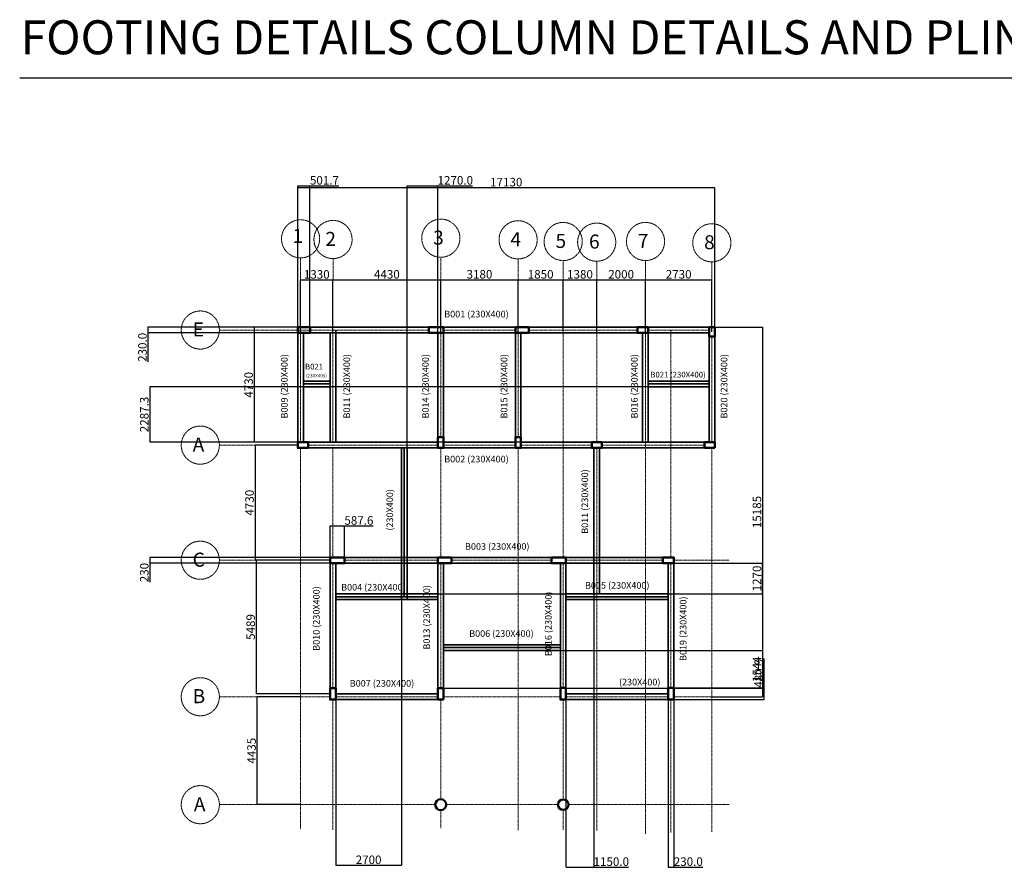
# Model space of a CAD drawing. Units: millimetres. Extents: x -2405 to 73447, y 417 to 55353.
# Tile 2 of 3: x -2405 to 38054, y 20479 to 55353. Entities that reach past the tile are written whole.
import ezdxf

# ---------------------------------------------------------------- set-up
doc = ezdxf.new("R2010")
doc.units = ezdxf.units.MM
doc.linetypes.add('CENTER', pattern=[50.8, 31.75, -6.35, 6.35, -6.35])
for name, color, linetype, lineweight in [('S-ANNO-DIMS', 2, 'Continuous', 18), ('S-ANNO-TEXT', 7, 'Continuous', 25), ('S-BEAM', 7, 'Continuous', 35), ('S-COLS', 4, 'Continuous', 50), ('S-GRID', 1, 'CENTER', 18)]:
    doc.layers.add(name, color=color, linetype=linetype, lineweight=lineweight)
doc.styles.get("Standard").update_dxf_attribs({"font": 'arial.ttf'})
doc.dimstyles.new('ISO-25', dxfattribs={"dimtxt": 350, "dimasz": 2.5, "dimexe": 1.25, "dimexo": 0.625, "dimtad": 1, "dimdec": 0, "dimtxsty": 'Standard', "dimcen": 2.5, "dimadec": 0, "dimazin": 0, "dimtfac": 1, "dimtdec": 0, "dimtmove": 0, "dimatfit": 3, "dimfxl": 1, "dimarcsym": 0})

# ---------------------------------------------------------------- blocks, each defined once
blk = doc.blocks.new('*D1')
at = {"layer": 'Defpoints', "color": 0, "transparency": 16777216}
for p in [(9023, 42715), (7229, 37985), (9023, 37985)]:
    blk.add_point(p, dxfattribs=at)
at = {"layer": 'S-ANNO-DIMS', "color": 0, "lineweight": -2, "transparency": 16777216}
for p, q in [((9022, 42715), (7227, 42715)), ((7229, 42712), (7229, 37987)), ((9022, 37985), (7227, 37985))]:
    blk.add_line(p, q, dxfattribs=at)
at = {"layer": 'S-ANNO-DIMS', "color": 0, "transparency": 16777216}
for points in [[(7228, 42712), (7229, 42712), (7229, 42715)], [(7228, 37987), (7229, 37987), (7229, 37985)]]:
    blk.add_solid(points, dxfattribs=at)
at = {"layer": 'S-ANNO-DIMS', "color": 0, "transparency": 16777216, "insert": (7049, 40350), "char_height": 350, "attachment_point": 5, "rotation": 90}
blk.add_mtext('4730', dxfattribs=at)
blk = doc.blocks.new('*D2')
at = {"layer": 'Defpoints', "color": 0, "transparency": 16777216}
for p in [(9023, 37870), (7265, 33140), (9138, 33140)]:
    blk.add_point(p, dxfattribs=at)
at = {"layer": 'S-ANNO-DIMS', "color": 0, "lineweight": -2, "transparency": 16777216}
for p, q in [((9022, 37870), (7263, 37870)), ((7265, 37867), (7265, 33142)), ((9137, 33140), (7263, 33140))]:
    blk.add_line(p, q, dxfattribs=at)
at = {"layer": 'S-ANNO-DIMS', "color": 0, "transparency": 16777216}
for points in [[(7264, 37867), (7265, 37867), (7265, 37870)], [(7264, 33142), (7265, 33142), (7265, 33140)]]:
    blk.add_solid(points, dxfattribs=at)
at = {"layer": 'S-ANNO-DIMS', "color": 0, "transparency": 16777216, "insert": (7085, 35505), "char_height": 350, "attachment_point": 5, "rotation": 90}
blk.add_mtext('4730', dxfattribs=at)
blk = doc.blocks.new('*D3')
at = {"layer": 'Defpoints', "color": 0, "transparency": 16777216}
for p in [(10353, 33140), (7309, 27651), (10353, 27651)]:
    blk.add_point(p, dxfattribs=at)
at = {"layer": 'S-ANNO-DIMS', "color": 0, "lineweight": -2, "transparency": 16777216}
for p, q in [((10352, 33140), (7308, 33140)), ((7309, 33137), (7309, 27654)), ((10352, 27651), (7308, 27651))]:
    blk.add_line(p, q, dxfattribs=at)
at = {"layer": 'S-ANNO-DIMS', "color": 0, "transparency": 16777216}
for points in [[(7309, 33137), (7310, 33137), (7309, 33140)], [(7309, 27654), (7310, 27654), (7309, 27651)]]:
    blk.add_solid(points, dxfattribs=at)
at = {"layer": 'S-ANNO-DIMS', "color": 0, "transparency": 16777216, "insert": (7130, 30396), "char_height": 350, "attachment_point": 5, "rotation": 90}
blk.add_mtext('5489', dxfattribs=at)
blk = doc.blocks.new('*D4')
at = {"layer": 'Defpoints', "color": 0, "transparency": 16777216}
for p in [(9138, 27530), (7345, 23095), (9138, 23095)]:
    blk.add_point(p, dxfattribs=at)
at = {"layer": 'S-ANNO-DIMS', "color": 0, "lineweight": -2, "transparency": 16777216}
for p, q in [((9137, 27530), (7344, 27530)), ((7345, 27527), (7345, 23097)), ((9137, 23095), (7344, 23095))]:
    blk.add_line(p, q, dxfattribs=at)
at = {"layer": 'S-ANNO-DIMS', "color": 0, "transparency": 16777216}
for points in [[(7345, 27527), (7346, 27527), (7345, 27530)], [(7345, 23097), (7346, 23097), (7345, 23095)]]:
    blk.add_solid(points, dxfattribs=at)
at = {"layer": 'S-ANNO-DIMS', "color": 0, "transparency": 16777216, "insert": (7166, 25312), "char_height": 350, "attachment_point": 5, "rotation": 90}
blk.add_mtext('4435', dxfattribs=at)
blk = doc.blocks.new('*D5')
at = {"layer": 'Defpoints', "color": 0, "transparency": 16777216}
for p in [(10468, 44661), (9138, 42485), (10468, 42485)]:
    blk.add_point(p, dxfattribs=at)
at = {"layer": 'S-ANNO-DIMS', "color": 0, "lineweight": -2, "transparency": 16777216}
for p, q in [((9138, 42486), (9138, 44662)), ((9140, 44661), (10465, 44661)), ((10468, 42486), (10468, 44662))]:
    blk.add_line(p, q, dxfattribs=at)
at = {"layer": 'S-ANNO-DIMS', "color": 0, "transparency": 16777216}
for points in [[(9140, 44662), (9140, 44661), (9138, 44661)], [(10465, 44662), (10465, 44661), (10468, 44661)]]:
    blk.add_solid(points, dxfattribs=at)
at = {"layer": 'S-ANNO-DIMS', "color": 0, "transparency": 16777216, "insert": (9803, 44841), "char_height": 350, "attachment_point": 5}
blk.add_mtext('1330', dxfattribs=at)
blk = doc.blocks.new('*D6')
at = {"layer": 'Defpoints', "color": 0, "transparency": 16777216}
for p in [(14898, 44665), (10468, 42485), (14898, 42485)]:
    blk.add_point(p, dxfattribs=at)
at = {"layer": 'S-ANNO-DIMS', "color": 0, "lineweight": -2, "transparency": 16777216}
for p, q in [((10468, 42486), (10468, 44666)), ((10470, 44665), (14895, 44665)), ((14898, 42486), (14898, 44666))]:
    blk.add_line(p, q, dxfattribs=at)
at = {"layer": 'S-ANNO-DIMS', "color": 0, "transparency": 16777216}
for points in [[(10470, 44665), (10470, 44664), (10468, 44665)], [(14895, 44665), (14895, 44664), (14898, 44665)]]:
    blk.add_solid(points, dxfattribs=at)
at = {"layer": 'S-ANNO-DIMS', "color": 0, "transparency": 16777216, "insert": (12683, 44844), "char_height": 350, "attachment_point": 5}
blk.add_mtext('4430', dxfattribs=at)
blk = doc.blocks.new('*D7')
at = {"layer": 'Defpoints', "color": 0, "transparency": 16777216}
for p in [(18078, 44666), (14898, 42485), (18078, 42485)]:
    blk.add_point(p, dxfattribs=at)
at = {"layer": 'S-ANNO-DIMS', "color": 0, "lineweight": -2, "transparency": 16777216}
for p, q in [((14898, 42486), (14898, 44667)), ((14900, 44666), (18075, 44666)), ((18078, 42486), (18078, 44667))]:
    blk.add_line(p, q, dxfattribs=at)
at = {"layer": 'S-ANNO-DIMS', "color": 0, "transparency": 16777216}
for points in [[(14900, 44667), (14900, 44666), (14898, 44666)], [(18075, 44667), (18075, 44666), (18078, 44666)]]:
    blk.add_solid(points, dxfattribs=at)
at = {"layer": 'S-ANNO-DIMS', "color": 0, "transparency": 16777216, "insert": (16488, 44846), "char_height": 350, "attachment_point": 5}
blk.add_mtext('3180', dxfattribs=at)
blk = doc.blocks.new('*D8')
at = {"layer": 'Defpoints', "color": 0, "transparency": 16777216}
for p in [(19928, 44666), (18078, 42485), (19928, 42600)]:
    blk.add_point(p, dxfattribs=at)
at = {"layer": 'S-ANNO-DIMS', "color": 0, "lineweight": -2, "transparency": 16777216}
for p, q in [((18078, 42486), (18078, 44667)), ((18080, 44666), (19925, 44666)), ((19928, 42601), (19928, 44667))]:
    blk.add_line(p, q, dxfattribs=at)
at = {"layer": 'S-ANNO-DIMS', "color": 0, "transparency": 16777216}
for points in [[(18080, 44666), (18080, 44665), (18078, 44666)], [(19925, 44666), (19925, 44665), (19928, 44666)]]:
    blk.add_solid(points, dxfattribs=at)
at = {"layer": 'S-ANNO-DIMS', "color": 0, "transparency": 16777216, "insert": (19003, 44845), "char_height": 350, "attachment_point": 5}
blk.add_mtext('1850', dxfattribs=at)
blk = doc.blocks.new('*D9')
at = {"layer": 'Defpoints', "color": 0, "transparency": 16777216}
for p in [(21308, 44666), (19928, 42600), (21308, 42485)]:
    blk.add_point(p, dxfattribs=at)
at = {"layer": 'S-ANNO-DIMS', "color": 0, "lineweight": -2, "transparency": 16777216}
for p, q in [((19928, 42601), (19928, 44667)), ((19930, 44666), (21305, 44666)), ((21308, 42486), (21308, 44667))]:
    blk.add_line(p, q, dxfattribs=at)
at = {"layer": 'S-ANNO-DIMS', "color": 0, "transparency": 16777216}
for points in [[(19930, 44666), (19930, 44665), (19928, 44666)], [(21305, 44666), (21305, 44665), (21308, 44666)]]:
    blk.add_solid(points, dxfattribs=at)
at = {"layer": 'S-ANNO-DIMS', "color": 0, "transparency": 16777216, "insert": (20618, 44845), "char_height": 350, "attachment_point": 5}
blk.add_mtext('1380', dxfattribs=at)
blk = doc.blocks.new('*D10')
at = {"layer": 'Defpoints', "color": 0, "transparency": 16777216}
for p in [(23308, 44665), (21308, 42600), (23308, 42485)]:
    blk.add_point(p, dxfattribs=at)
at = {"layer": 'S-ANNO-DIMS', "color": 0, "lineweight": -2, "transparency": 16777216}
for p, q in [((21308, 42601), (21308, 44667)), ((21310, 44665), (23305, 44665)), ((23308, 42486), (23308, 44667))]:
    blk.add_line(p, q, dxfattribs=at)
at = {"layer": 'S-ANNO-DIMS', "color": 0, "transparency": 16777216}
for points in [[(21310, 44666), (21310, 44665), (21308, 44665)], [(23305, 44666), (23305, 44665), (23308, 44665)]]:
    blk.add_solid(points, dxfattribs=at)
at = {"layer": 'S-ANNO-DIMS', "color": 0, "transparency": 16777216, "insert": (22308, 44845), "char_height": 350, "attachment_point": 5}
blk.add_mtext('2000', dxfattribs=at)
blk = doc.blocks.new('*D11')
at = {"layer": 'Defpoints', "color": 0, "transparency": 16777216}
for p in [(26038, 44666), (23308, 42485), (26038, 42525)]:
    blk.add_point(p, dxfattribs=at)
at = {"layer": 'S-ANNO-DIMS', "color": 0, "lineweight": -2, "transparency": 16777216}
for p, q in [((23308, 42486), (23308, 44667)), ((23310, 44666), (26035, 44666)), ((26038, 42525), (26038, 44667))]:
    blk.add_line(p, q, dxfattribs=at)
at = {"layer": 'S-ANNO-DIMS', "color": 0, "transparency": 16777216}
for points in [[(23310, 44666), (23310, 44665), (23308, 44666)], [(26035, 44666), (26035, 44665), (26038, 44666)]]:
    blk.add_solid(points, dxfattribs=at)
at = {"layer": 'S-ANNO-DIMS', "color": 0, "transparency": 16777216, "insert": (24673, 44845), "char_height": 350, "attachment_point": 5}
blk.add_mtext('2730', dxfattribs=at)
blk = doc.blocks.new('*D14')
at = {"layer": 'Defpoints', "color": 0, "transparency": 16777216}
for p in [(26153, 48453), (9023, 42715), (26153, 42715)]:
    blk.add_point(p, dxfattribs=at)
at = {"layer": 'S-ANNO-DIMS', "color": 0, "lineweight": -2, "transparency": 16777216}
for p, q in [((9023, 42716), (9023, 48454)), ((9025, 48453), (26150, 48453)), ((26153, 42716), (26153, 48454))]:
    blk.add_line(p, q, dxfattribs=at)
at = {"layer": 'S-ANNO-DIMS', "color": 0, "transparency": 16777216}
for points in [[(9025, 48453), (9025, 48452), (9023, 48453)], [(26150, 48453), (26150, 48452), (26153, 48453)]]:
    blk.add_solid(points, dxfattribs=at)
at = {"layer": 'S-ANNO-DIMS', "color": 0, "transparency": 16777216, "insert": (17588, 48632), "char_height": 350, "attachment_point": 5}
blk.add_mtext('17130', dxfattribs=at)
blk = doc.blocks.new('*D15')
at = {"layer": 'Defpoints', "color": 0, "transparency": 16777216}
for p in [(26153, 42715), (26038, 27530), (28113, 27530)]:
    blk.add_point(p, dxfattribs=at)
at = {"layer": 'S-ANNO-DIMS', "color": 0, "lineweight": -2, "transparency": 16777216}
for p, q in [((26153, 42715), (28115, 42715)), ((28113, 42712), (28113, 27532)), ((26038, 27530), (28115, 27530))]:
    blk.add_line(p, q, dxfattribs=at)
at = {"layer": 'S-ANNO-DIMS', "color": 0, "transparency": 16777216}
for points in [[(28113, 42712), (28114, 42712), (28113, 42715)], [(28113, 27532), (28114, 27532), (28113, 27530)]]:
    blk.add_solid(points, dxfattribs=at)
at = {"layer": 'S-ANNO-DIMS', "color": 0, "transparency": 16777216, "insert": (27934, 35122), "char_height": 350, "attachment_point": 5, "rotation": 90}
blk.add_mtext('15185', dxfattribs=at)
blk = doc.blocks.new('*D16')
at = {"layer": 'Defpoints', "color": 0, "transparency": 16777216}
for p in [(10940, 34550), (10353, 33255), (10940, 33255)]:
    blk.add_point(p, dxfattribs=at)
at = {"layer": 'S-ANNO-DIMS', "color": 0, "lineweight": -2, "transparency": 16777216}
for p, q in [((10353, 33256), (10353, 34551)), ((10355, 34550), (10938, 34550)), ((10940, 33256), (10940, 34551)), ((10940, 34550), (12125, 34550))]:
    blk.add_line(p, q, dxfattribs=at)
at = {"layer": 'S-ANNO-DIMS', "color": 0, "transparency": 16777216}
for points in [[(10355, 34550), (10355, 34550), (10353, 34550)], [(10938, 34550), (10938, 34550), (10940, 34550)]]:
    blk.add_solid(points, dxfattribs=at)
at = {"layer": 'S-ANNO-DIMS', "color": 0, "transparency": 16777216, "insert": (11534, 34729), "char_height": 350, "attachment_point": 5}
blk.add_mtext('587.6', dxfattribs=at)
blk = doc.blocks.new('*D17')
at = {"layer": 'Defpoints', "color": 0, "transparency": 16777216}
for p in [(14783, 33255), (2939, 33025), (14783, 33025)]:
    blk.add_point(p, dxfattribs=at)
at = {"layer": 'S-ANNO-DIMS', "color": 0, "lineweight": -2, "transparency": 16777216}
for p, q in [((14782, 33255), (2938, 33255)), ((2939, 33252), (2939, 33027)), ((14782, 33025), (2938, 33025)), ((2939, 33025), (2939, 32243))]:
    blk.add_line(p, q, dxfattribs=at)
at = {"layer": 'S-ANNO-DIMS', "color": 0, "transparency": 16777216}
for points in [[(2939, 33252), (2940, 33252), (2939, 33255)], [(2939, 33027), (2940, 33027), (2939, 33025)]]:
    blk.add_solid(points, dxfattribs=at)
at = {"layer": 'S-ANNO-DIMS', "color": 0, "transparency": 16777216, "insert": (2760, 32633), "char_height": 350, "attachment_point": 5, "rotation": 90}
blk.add_mtext('230', dxfattribs=at)
blk = doc.blocks.new('*D18')
at = {"layer": 'Defpoints', "color": 0, "transparency": 16777216}
for p in [(10583, 31525), (13283, 31525), (13283, 20604)]:
    blk.add_point(p, dxfattribs=at)
at = {"layer": 'S-ANNO-DIMS', "color": 0, "lineweight": -2, "transparency": 16777216}
for p, q in [((10583, 31524), (10583, 20603)), ((13283, 31524), (13283, 20603)), ((10585, 20604), (13280, 20604))]:
    blk.add_line(p, q, dxfattribs=at)
at = {"layer": 'S-ANNO-DIMS', "color": 0, "transparency": 16777216}
for points in [[(10585, 20605), (10585, 20604), (10583, 20604)], [(13280, 20605), (13280, 20604), (13283, 20604)]]:
    blk.add_solid(points, dxfattribs=at)
at = {"layer": 'S-ANNO-DIMS', "color": 0, "transparency": 16777216, "insert": (11933, 20784), "char_height": 350, "attachment_point": 5}
blk.add_mtext('2700', dxfattribs=at)
blk = doc.blocks.new('*D19')
at = {"layer": 'Defpoints', "color": 0, "transparency": 16777216}
for p in [(14783, 33025), (28113, 33025), (14783, 31755)]:
    blk.add_point(p, dxfattribs=at)
at = {"layer": 'S-ANNO-DIMS', "color": 0, "lineweight": -2, "transparency": 16777216}
for p, q in [((14783, 33025), (28115, 33025)), ((28113, 31757), (28113, 33022)), ((14783, 31755), (28115, 31755))]:
    blk.add_line(p, q, dxfattribs=at)
at = {"layer": 'S-ANNO-DIMS', "color": 0, "transparency": 16777216}
for points in [[(28113, 33022), (28114, 33022), (28113, 33025)], [(28113, 31757), (28114, 31757), (28113, 31755)]]:
    blk.add_solid(points, dxfattribs=at)
at = {"layer": 'S-ANNO-DIMS', "color": 0, "transparency": 16777216, "insert": (27934, 32390), "char_height": 350, "attachment_point": 5, "rotation": 90}
blk.add_mtext('1270', dxfattribs=at)
blk = doc.blocks.new('*D20')
at = {"layer": 'Defpoints', "color": 0, "transparency": 16777216}
for p in [(15013, 29432), (15013, 27888), (28113, 27888)]:
    blk.add_point(p, dxfattribs=at)
at = {"layer": 'S-ANNO-DIMS', "color": 0, "lineweight": -2, "transparency": 16777216}
for p, q in [((15013, 29432), (28115, 29432)), ((28113, 29429), (28113, 27890)), ((15013, 27888), (28115, 27888))]:
    blk.add_line(p, q, dxfattribs=at)
at = {"layer": 'S-ANNO-DIMS', "color": 0, "transparency": 16777216}
for points in [[(28113, 29429), (28114, 29429), (28113, 29432)], [(28113, 27890), (28114, 27890), (28113, 27888)]]:
    blk.add_solid(points, dxfattribs=at)
at = {"layer": 'S-ANNO-DIMS', "color": 0, "transparency": 16777216, "insert": (27934, 28660), "char_height": 350, "attachment_point": 5, "rotation": 90}
blk.add_mtext('1544', dxfattribs=at)
blk = doc.blocks.new('*D21')
at = {"layer": 'Defpoints', "color": 0, "transparency": 16777216}
for p in [(25923, 40272), (2939, 37985), (25923, 37985)]:
    blk.add_point(p, dxfattribs=at)
at = {"layer": 'S-ANNO-DIMS', "color": 0, "lineweight": -2, "transparency": 16777216}
for p, q in [((25922, 40272), (2938, 40272)), ((2939, 40270), (2939, 37987)), ((25922, 37985), (2938, 37985))]:
    blk.add_line(p, q, dxfattribs=at)
at = {"layer": 'S-ANNO-DIMS', "color": 0, "transparency": 16777216}
for points in [[(2939, 40270), (2940, 40270), (2939, 40272)], [(2939, 37987), (2940, 37987), (2939, 37985)]]:
    blk.add_solid(points, dxfattribs=at)
at = {"layer": 'S-ANNO-DIMS', "color": 0, "transparency": 16777216, "insert": (2760, 39129), "char_height": 350, "attachment_point": 5, "rotation": 90}
blk.add_mtext('2287.3', dxfattribs=at)
blk = doc.blocks.new('*D22')
at = {"layer": 'Defpoints', "color": 0, "transparency": 16777216}
for p in [(24358, 33025), (28113, 33025), (24243, 31755)]:
    blk.add_point(p, dxfattribs=at)
at = {"layer": 'S-ANNO-DIMS', "color": 0, "lineweight": -2, "transparency": 16777216}
for p, q in [((24358, 33025), (28115, 33025)), ((28113, 31757), (28113, 33022)), ((24243, 31755), (28115, 31755))]:
    blk.add_line(p, q, dxfattribs=at)
at = {"layer": 'S-ANNO-DIMS', "color": 0, "transparency": 16777216}
for points in [[(28113, 33022), (28114, 33022), (28113, 33025)], [(28113, 31757), (28114, 31757), (28113, 31755)]]:
    blk.add_solid(points, dxfattribs=at)
at = {"layer": 'S-ANNO-DIMS', "color": 0, "transparency": 16777216, "insert": (27934, 32390), "char_height": 350, "attachment_point": 5, "rotation": 90}
blk.add_mtext('1270', dxfattribs=at)
blk = doc.blocks.new('*D40')
at = {"layer": 'Defpoints', "color": 0, "transparency": 16777216}
for p in [(9524, 48528), (9023, 42715), (9524, 42715)]:
    blk.add_point(p, dxfattribs=at)
at = {"layer": 'S-ANNO-DIMS', "color": 0, "lineweight": -2, "transparency": 16777216}
for p, q in [((9023, 42716), (9023, 48529)), ((9025, 48528), (9522, 48528)), ((9524, 42716), (9524, 48529)), ((9524, 48528), (10709, 48528))]:
    blk.add_line(p, q, dxfattribs=at)
at = {"layer": 'S-ANNO-DIMS', "color": 0, "transparency": 16777216}
for points in [[(9025, 48528), (9025, 48527), (9023, 48528)], [(9522, 48528), (9522, 48527), (9524, 48528)]]:
    blk.add_solid(points, dxfattribs=at)
at = {"layer": 'S-ANNO-DIMS', "color": 0, "transparency": 16777216, "insert": (10118, 48707), "char_height": 350, "attachment_point": 5}
blk.add_mtext('501.7', dxfattribs=at)
blk = doc.blocks.new('*D41')
at = {"layer": 'Defpoints', "color": 0, "transparency": 16777216}
for p in [(2864, 42485), (9023, 42715), (9023, 42485)]:
    blk.add_point(p, dxfattribs=at)
at = {"layer": 'S-ANNO-DIMS', "color": 0, "lineweight": -2, "transparency": 16777216}
for p, q in [((9022, 42715), (2863, 42715)), ((9022, 42485), (2863, 42485)), ((2864, 42712), (2864, 42487)), ((2864, 42485), (2864, 41295))]:
    blk.add_line(p, q, dxfattribs=at)
at = {"layer": 'S-ANNO-DIMS', "color": 0, "transparency": 16777216}
for points in [[(2864, 42712), (2865, 42712), (2864, 42715)], [(2864, 42487), (2865, 42487), (2864, 42485)]]:
    blk.add_solid(points, dxfattribs=at)
at = {"layer": 'S-ANNO-DIMS', "color": 0, "transparency": 16777216, "insert": (2685, 41889), "char_height": 350, "attachment_point": 5, "rotation": 90}
blk.add_mtext('230.0', dxfattribs=at)
blk = doc.blocks.new('*D42')
at = {"layer": 'Defpoints', "color": 0, "transparency": 16777216}
for p in [(24473, 27896), (28188, 27896), (24473, 27415)]:
    blk.add_point(p, dxfattribs=at)
at = {"layer": 'S-ANNO-DIMS', "color": 0, "lineweight": -2, "transparency": 16777216}
for p, q in [((28188, 27896), (28188, 29095)), ((24473, 27896), (28190, 27896)), ((28188, 27417), (28188, 27893)), ((24473, 27415), (28190, 27415))]:
    blk.add_line(p, q, dxfattribs=at)
at = {"layer": 'S-ANNO-DIMS', "color": 0, "transparency": 16777216}
for points in [[(28188, 27893), (28189, 27893), (28188, 27896)], [(28188, 27417), (28189, 27417), (28188, 27415)]]:
    blk.add_solid(points, dxfattribs=at)
at = {"layer": 'S-ANNO-DIMS', "color": 0, "transparency": 16777216, "insert": (28009, 28497), "char_height": 350, "attachment_point": 5, "rotation": 90}
blk.add_mtext('480.9', dxfattribs=at)
blk = doc.blocks.new('*D43')
at = {"layer": 'Defpoints', "color": 0, "transparency": 16777216}
for p in [(24243, 27415), (24473, 27415), (24473, 20529)]:
    blk.add_point(p, dxfattribs=at)
at = {"layer": 'S-ANNO-DIMS', "color": 0, "lineweight": -2, "transparency": 16777216}
for p, q in [((24243, 27414), (24243, 20528)), ((24473, 27414), (24473, 20528)), ((24245, 20529), (24470, 20529)), ((24473, 20529), (25662, 20529))]:
    blk.add_line(p, q, dxfattribs=at)
at = {"layer": 'S-ANNO-DIMS', "color": 0, "transparency": 16777216}
for points in [[(24245, 20530), (24245, 20529), (24243, 20529)], [(24470, 20530), (24470, 20529), (24473, 20529)]]:
    blk.add_solid(points, dxfattribs=at)
at = {"layer": 'S-ANNO-DIMS', "color": 0, "transparency": 16777216, "insert": (25069, 20709), "char_height": 350, "attachment_point": 5}
blk.add_mtext('230.0', dxfattribs=at)
blk = doc.blocks.new('*D44')
at = {"layer": 'Defpoints', "color": 0, "transparency": 16777216}
for p in [(14783, 48528), (13513, 37755), (14783, 37755)]:
    blk.add_point(p, dxfattribs=at)
at = {"layer": 'S-ANNO-DIMS', "color": 0, "lineweight": -2, "transparency": 16777216}
for p, q in [((13513, 37756), (13513, 48529)), ((13515, 48528), (14780, 48528)), ((14783, 37756), (14783, 48529)), ((14783, 48528), (16205, 48528))]:
    blk.add_line(p, q, dxfattribs=at)
at = {"layer": 'S-ANNO-DIMS', "color": 0, "transparency": 16777216}
for points in [[(13515, 48528), (13515, 48527), (13513, 48528)], [(14780, 48528), (14780, 48527), (14783, 48528)]]:
    blk.add_solid(points, dxfattribs=at)
at = {"layer": 'S-ANNO-DIMS', "color": 0, "transparency": 16777216, "insert": (15495, 48707), "char_height": 350, "attachment_point": 5}
blk.add_mtext('1270.0', dxfattribs=at)
blk = doc.blocks.new('*D45')
at = {"layer": 'Defpoints', "color": 0, "transparency": 16777216}
for p in [(20043, 31755), (21193, 31755), (21193, 20529)]:
    blk.add_point(p, dxfattribs=at)
at = {"layer": 'S-ANNO-DIMS', "color": 0, "lineweight": -2, "transparency": 16777216}
for p, q in [((20043, 31754), (20043, 20528)), ((21193, 31754), (21193, 20528)), ((20045, 20529), (21190, 20529)), ((21193, 20529), (22615, 20529))]:
    blk.add_line(p, q, dxfattribs=at)
at = {"layer": 'S-ANNO-DIMS', "color": 0, "transparency": 16777216}
for points in [[(20045, 20530), (20045, 20529), (20043, 20529)], [(21190, 20530), (21190, 20529), (21193, 20529)]]:
    blk.add_solid(points, dxfattribs=at)
at = {"layer": 'S-ANNO-DIMS', "color": 0, "transparency": 16777216, "insert": (21905, 20709), "char_height": 350, "attachment_point": 5}
blk.add_mtext('1150.0', dxfattribs=at)

msp = doc.modelspace()

# ---------------------------------------------------------------- linework, layer by layer
at = {"layer": 'S-ANNO-TEXT'}
msp.add_line((-2404.637, 52969.195), (57098.008, 52969.195), dxfattribs=at)
at = {"layer": 'S-BEAM'}
for p, q in [((9022.761, 42599.973), (9022.761, 42714.973)), ((9022.761, 42714.973), (9137.761, 42714.973)), ((9022.761, 42599.973), (9022.761, 37754.973)), ((9022.761, 42484.973), (10467.761, 42484.973)), ((9137.761, 42714.973), (10467.761, 42714.973)), ((9252.761, 42484.973), (9252.761, 37984.973)), ((10352.761, 42484.973), (10352.761, 37984.973)), ((10467.761, 42714.973), (14897.761, 42714.973)), ((10467.761, 42484.973), (14897.761, 42484.973)), ((10582.761, 42599.973), (10582.761, 37984.973)), ((14782.761, 42484.973), (14782.761, 37754.973)), ((14897.761, 42714.973), (18077.761, 42714.973)), ((14897.761, 42484.973), (18077.761, 42484.973)), ((15012.761, 42484.973), (15012.761, 37754.973)), ((17962.761, 42714.973), (17962.761, 37754.973)), ((18077.761, 42714.973), (19927.761, 42714.973)), ((18077.761, 42484.973), (19927.761, 42484.973)), ((18192.761, 42484.973), (18192.761, 37754.973)), ((19927.761, 42714.973), (21307.761, 42714.973)), ((19927.761, 42484.973), (21307.761, 42484.973)), ((21307.761, 42714.973), (23307.761, 42714.973)), ((21307.761, 42484.973), (23307.761, 42484.973)), ((23192.761, 42484.973), (23192.761, 37984.973)), ((23307.761, 42714.973), (24357.761, 42714.973)), ((23307.761, 42484.973), (24357.761, 42484.973)), ((23422.761, 42599.973), (23422.761, 37984.973)), ((24357.761, 42714.973), (26037.761, 42714.973)), ((24357.761, 42484.973), (25922.761, 42484.973)), ((25922.761, 37984.973), (25922.761, 42599.973)), ((26152.761, 42714.973), (26037.761, 42714.973)), ((26152.761, 42599.973), (26152.761, 42714.973)), ((26152.761, 37754.973), (26152.761, 42599.973)), ((9252.761, 40502.295), (10352.761, 40502.295)), ((23422.761, 40502.295), (25922.761, 40502.295)), ((9252.761, 40387.295), (10352.761, 40387.295)), ((9252.761, 40272.295), (10352.761, 40272.295)), ((23422.761, 40387.295), (25922.761, 40387.295)), ((23422.761, 40272.295), (25922.761, 40272.295)), ((9022.761, 37984.973), (10467.761, 37984.973)), ((9022.761, 37754.973), (10467.761, 37754.973)), ((10467.761, 37984.973), (14782.761, 37984.973)), ((10467.761, 37754.973), (14897.761, 37754.973)), ((13282.761, 37754.973), (13282.761, 31524.973)), ((13397.761, 37754.973), (13397.761, 31639.973)), ((13512.761, 37754.973), (13512.761, 31524.973)), ((14897.761, 37754.973), (19927.761, 37754.973)), ((15012.761, 37984.973), (17962.761, 37984.973)), ((18192.761, 37984.973), (19927.761, 37984.973)), ((19927.761, 37984.973), (21307.761, 37984.973)), ((19927.761, 37754.973), (21307.761, 37754.973)), ((21192.761, 37754.973), (21192.761, 31754.973)), ((21307.761, 37984.973), (23307.761, 37984.973)), ((21307.761, 37754.973), (23307.761, 37754.973)), ((21422.761, 37754.973), (21422.761, 31754.973)), ((23307.761, 37984.973), (26152.761, 37984.973)), ((23307.761, 37754.973), (26152.761, 37754.973)), ((10352.761, 33254.973), (14897.761, 33254.973)), ((10352.761, 33254.973), (10352.761, 27414.973)), ((14782.761, 33254.973), (14782.761, 27414.973)), ((14897.761, 33254.973), (18077.761, 33254.973)), ((18077.761, 33254.973), (19927.761, 33254.973)), ((19812.761, 33254.973), (21307.761, 33254.973)), ((20042.761, 33254.973), (20042.761, 27529.973)), ((21307.761, 33254.973), (23307.761, 33254.973)), ((23307.761, 33254.973), (24472.761, 33254.973)), ((24472.761, 33254.973), (24472.761, 27414.973)), ((10352.761, 33024.973), (14897.761, 33024.973)), ((10582.761, 33024.973), (10582.761, 27414.973)), ((14897.761, 33024.973), (18077.761, 33024.973)), ((15012.761, 33024.973), (15012.761, 27414.973)), ((18077.761, 33024.973), (19927.761, 33024.973)), ((19812.761, 33024.973), (21307.761, 33024.973)), ((19812.761, 33024.973), (19812.761, 27529.973)), ((21307.761, 33024.973), (23307.761, 33024.973)), ((23307.761, 33024.973), (24472.761, 33024.973)), ((24242.761, 33024.973), (24242.761, 27414.973)), ((10582.761, 31754.973), (14782.761, 31754.973)), ((10582.761, 31639.973), (14782.761, 31639.973)), ((20042.761, 31754.973), (21307.761, 31754.973)), ((20042.761, 31639.973), (21307.761, 31639.973)), ((21307.761, 31754.973), (23307.761, 31754.973)), ((21307.761, 31639.973), (23307.761, 31639.973)), ((23307.761, 31754.973), (24242.761, 31754.973)), ((23307.761, 31639.973), (24242.761, 31639.973)), ((10582.761, 31524.973), (14782.761, 31524.973)), ((20042.761, 31524.973), (21307.761, 31524.973)), ((21307.761, 31524.973), (23307.761, 31524.973)), ((23307.761, 31524.973), (24242.761, 31524.973)), ((15012.761, 29661.949), (19812.761, 29661.949)), ((15012.761, 29546.949), (19812.761, 29546.949)), ((15012.761, 29431.949), (19812.761, 29431.949)), ((10582.761, 27644.973), (14782.761, 27644.973)), ((20042.761, 27644.973), (23307.761, 27644.973)), ((23307.761, 27644.973), (24242.761, 27644.973)), ((10352.761, 27414.973), (15012.761, 27414.973)), ((19927.761, 27414.973), (23307.761, 27414.973)), ((23307.761, 27414.973), (24472.761, 27414.973))]:
    msp.add_line(p, q, dxfattribs=at)
at = {"layer": 'S-COLS'}
for points in [[(9022.761, 42714.973), (9524.48, 42714.973), (9524.48, 42484.973), (9022.761, 42484.973)], [(15012.761, 42484.973), (14411.901, 42484.973), (14411.901, 42714.973), (15012.761, 42714.973)], [(17962.761, 42484.973), (18518.958, 42484.973), (18518.958, 42714.973), (17962.761, 42714.973)], [(23422.761, 42484.973), (22981.975, 42484.973), (22981.975, 42714.973), (23422.761, 42714.973)], [(25922.761, 42714.973), (26152.761, 42714.973), (26152.761, 42334.257), (25922.761, 42334.257)], [(14782.761, 38201.603), (15012.761, 38201.603), (15012.761, 37754.973), (14782.761, 37754.973)], [(17962.761, 38195.273), (18192.761, 38195.273), (18192.761, 37754.973), (17962.761, 37754.973)], [(9022.761, 37984.973), (9448.304, 37984.973), (9448.304, 37754.973), (9022.761, 37754.973)], [(21099.782, 37984.973), (21521.553, 37984.973), (21521.553, 37754.973), (21099.782, 37754.973)], [(26152.761, 37754.973), (25741.095, 37754.973), (25741.095, 37984.973), (26152.761, 37984.973)], [(10352.761, 33254.973), (10940.339, 33254.973), (10940.339, 33024.973), (10352.761, 33024.973)], [(14782.761, 33254.973), (15336.251, 33254.973), (15336.251, 33024.973), (14782.761, 33024.973)], [(20042.761, 33024.973), (19448.458, 33024.973), (19448.458, 33254.973), (20042.761, 33254.973)], [(24472.761, 33024.973), (24025.178, 33024.973), (24025.178, 33254.973), (24472.761, 33254.973)], [(10582.761, 27414.973), (10352.761, 27414.973), (10352.761, 27887.842), (10582.761, 27887.842)], [(15012.761, 27414.973), (14782.761, 27414.973), (14782.761, 27887.842), (15012.761, 27887.842)], [(20042.761, 27414.973), (19812.761, 27414.973), (19812.761, 27890.006), (20042.761, 27890.006)], [(24472.761, 27414.973), (24242.761, 27414.973), (24242.761, 27895.844), (24472.761, 27895.844)]]:
    msp.add_lwpolyline(points, close=True, dxfattribs=at)
for centre, radius in [((14897.761, 23094.973), 224.403), ((19927.761, 23094.973), 214.907)]:
    msp.add_circle(centre, radius, dxfattribs=at)
at = {"layer": 'S-GRID'}
for p, q in [((9137.761, 44661.1), (9137.761, 45563.747)), ((10470.261, 44665.267), (10470.261, 45536.682)), ((14900.261, 44661.1), (14900.261, 45591.188)), ((18075.261, 44666.517), (18075.261, 45523.244)), ((19927.761, 44661.933), (19927.761, 45455.166)), ((21305.261, 44665.267), (21305.261, 45427.94)), ((23310.261, 44666.1), (23310.261, 45455.407)), ((26035.261, 44665.267), (26035.261, 45400.902)), ((9524.48, 42599.973), (5800.882, 42599.973)), ((9137.761, 42484.973), (9137.761, 37984.973)), ((9524.48, 42599.973), (10467.761, 42599.973)), ((10467.761, 42599.973), (14411.901, 42599.973)), ((10467.761, 42484.973), (10467.761, 37984.973)), ((14897.761, 42484.973), (14897.761, 38201.603)), ((15012.761, 42599.973), (17962.761, 42599.973)), ((18077.761, 42484.973), (18077.761, 38195.273)), ((18518.958, 42599.973), (19927.761, 42599.973)), ((19927.761, 42599.973), (21307.761, 42599.973)), ((19927.761, 42599.973), (19927.761, 33254.973)), ((21307.761, 42599.973), (22981.975, 42599.973)), ((21307.761, 42599.973), (21307.761, 37984.973)), ((23307.761, 42484.973), (23307.761, 21899.44)), ((23422.761, 42599.973), (24357.761, 42599.973)), ((24357.761, 42599.973), (25922.761, 42599.973)), ((24357.761, 42599.973), (24357.761, 33254.973)), ((26037.761, 37984.973), (26037.761, 42334.257)), ((5800.882, 37869.973), (9022.761, 37869.973)), ((9137.761, 37754.973), (9137.761, 33139.973)), ((9448.304, 37869.973), (10467.761, 37869.973)), ((10467.761, 37869.973), (14782.761, 37869.973)), ((10467.761, 37754.973), (10467.761, 33254.973)), ((14897.761, 37754.973), (14897.761, 33254.973)), ((15012.761, 37869.973), (17962.761, 37869.973)), ((18077.761, 37754.973), (18077.761, 22053.413)), ((18192.761, 37869.973), (19927.761, 37869.973)), ((19927.761, 37869.973), (21099.782, 37869.973)), ((21307.761, 37754.973), (21307.761, 22035.116)), ((21521.553, 37869.973), (23307.761, 37869.973)), ((23307.761, 37869.973), (25741.095, 37869.973)), ((26037.761, 33139.973), (26037.761, 37754.973)), ((5800.882, 33139.973), (10352.761, 33139.973)), ((9137.761, 33139.973), (9137.761, 27529.973)), ((10467.761, 33024.973), (10467.761, 27887.842)), ((10940.339, 33139.973), (14782.761, 33139.973)), ((14897.761, 33024.973), (14897.761, 27887.842)), ((15336.251, 33139.973), (18077.761, 33139.973)), ((18077.761, 33139.973), (19448.458, 33139.973)), ((19927.761, 33024.973), (19927.761, 27890.006)), ((20042.761, 33139.973), (21307.761, 33139.973)), ((21307.761, 33139.973), (23307.761, 33139.973)), ((23307.761, 33139.973), (24025.178, 33139.973)), ((24357.761, 33024.973), (24357.761, 27895.844)), ((24472.761, 33139.973), (26754.153, 33139.973)), ((26037.761, 27529.973), (26037.761, 33139.973)), ((5800.882, 27529.973), (10352.761, 27529.973)), ((9137.761, 27529.973), (9137.761, 22088.194)), ((10582.761, 27529.973), (14782.761, 27529.973)), ((15012.761, 27529.973), (18077.761, 27529.973)), ((18077.761, 27529.973), (19812.761, 27529.973)), ((20042.761, 27529.973), (21307.761, 27529.973)), ((21192.761, 27529.973), (23307.761, 27529.973)), ((23307.761, 27529.973), (24242.761, 27529.973)), ((24472.761, 27529.973), (26754.153, 27529.973)), ((26037.761, 21982.058), (26037.761, 27529.973)), ((10467.761, 27414.973), (10467.761, 22060.988)), ((14897.761, 27414.973), (14897.761, 23319.376)), ((19927.761, 27414.973), (19927.761, 23309.88)), ((24357.761, 27414.973), (24357.761, 21951.088)), ((5800.882, 23094.973), (10467.761, 23094.973)), ((10467.761, 23094.973), (14673.358, 23094.973)), ((15122.164, 23094.973), (18077.761, 23094.973)), ((18077.761, 23094.973), (19712.854, 23094.973)), ((20142.668, 23094.973), (21307.761, 23094.973)), ((21307.761, 23094.973), (23307.761, 23094.973)), ((23307.761, 23094.973), (26754.153, 23094.973)), ((14897.761, 22870.57), (14897.761, 22132.609)), ((19927.761, 22880.066), (19927.761, 22060.311))]:
    msp.add_line(p, q, dxfattribs=at)
for centre in [(9137.761, 46346.939), (10470.261, 46319.875), (14900.261, 46374.38), (18075.261, 46306.436), (19927.761, 46238.358), (21305.261, 46211.132), (23310.261, 46238.6), (26035.261, 46184.094), (5017.69, 42599.973), (5017.69, 37869.973), (5017.69, 33139.973), (5017.69, 27529.973), (5017.69, 23094.973)]:
    msp.add_circle(centre, 783.192, dxfattribs=at)

# ---------------------------------------------------------------- texts
at = {"layer": 'S-ANNO-TEXT'}
for s, height, p in [('FOOTING DETAILS COLUMN DETAILS AND PLINTH BEAM PLAN', 1397.07747, (-2368.288, 53931.557)), ('B001 (230X400)', 272.58037, (15040.076, 43117.808)), ('B021', 233.8995, (9320.154, 40978.849)), ('B021 (230X400)', 233.89945, (23508.649, 40649.956)), ('(230X400)', 137.2742, (9358.932, 40652.656)), ('B002 (230X400)', 272.58037, (15040.076, 37159.158)), ('B003 (230X400)', 272.58037, (15893.248, 33569.602)), ('B004 (230X400)', 272.58037, (10803.193, 31893.623)), ('B005 (230X400)', 272.58037, (20823.73, 31968.452)), ('B006 (230X400)', 272.58037, (16065.129, 29990.428)), ('B007 (230X400)', 272.58037, (11156.831, 27944.167)), (' (230X400)', 272.5804, (22137.353, 27995.312))]:
    msp.add_text(s, height=height, dxfattribs=at).set_placement(p)
for s, height, p in [('B009 (230X400)', 272.58037, (8607.461, 38964.771)), ('B011 (230X400)', 272.58037, (11171.345, 38964.771)), ('B014 (230X400)', 272.58037, (14406.867, 38964.771)), ('B015 (230X400)', 272.58037, (17634.42, 38964.771)), ('B016 (230X400)', 272.58037, (22989.233, 38964.771)), ('B020 (230X400)', 272.58037, (26675.681, 38964.771)), ('B011 (230X400)', 272.58037, (20953.966, 34227.121)), (' (230X400)', 272.5804, (12940.072, 34274.759)), ('B010 (230X400)', 272.58037, (9921.385, 29419.016)), ('B013 (230X400)', 272.58037, (14454.968, 29468.502)), ('B016 (230X400)', 272.58037, (19455.742, 29199.849)), ('B019 (230X400)', 272.58037, (24992.584, 28999.038))]:
    msp.add_text(s, height=height, rotation=90, dxfattribs=at).set_placement(p)
at = {"layer": 'S-GRID'}
for s, p in [('1', (8808.327, 46180.92)), ('2', (10153.958, 46055.433)), ('3', (14583.958, 46109.939)), ('4', (17758.958, 46041.995)), ('5', (19611.458, 45973.917)), ('6', (20988.958, 45946.691)), ('7', (22993.958, 45974.159)), ('8', (25718.958, 45919.653)), ('E', (4701.386, 42335.532)), ('A', (4701.386, 37605.532)), ('C', (4701.386, 32875.532)), ('B', (4701.386, 27265.532)), ('A', (4750.432, 22821.696))]:
    msp.add_text(s, height=576.596, dxfattribs=at).set_placement(p)

# ---------------------------------------------------------------- dimensions: what is measured, and where the dimension line sits
at = {"layer": 'S-ANNO-DIMS'}
for base, p1, p2, override, picture, middle in [((9524.48, 48527.573), (9022.761, 42714.973), (9524.48, 42714.973), {"dimdec": 1, "dimlfac": 1, "dimrnd": 0, "dimzin": 0, "dimdsep": 46, "dimlunit": 2}, '*D40', (10118.141, 48706.898)), ((26152.761, 48452.573), (9022.761, 42714.973), (26152.761, 42714.973), {"dimdec": 0, "dimlfac": 1, "dimrnd": 0, "dimzin": 0, "dimdsep": 46, "dimlunit": 2}, '*D14', (17587.761, 48632.017)), ((14782.761, 48527.573), (13512.761, 37754.973), (14782.761, 37754.973), {"dimdec": 1, "dimlfac": 1, "dimrnd": 0, "dimzin": 0, "dimdsep": 46, "dimlunit": 2}, '*D44', (15495.316, 48706.898)), ((10467.761, 44661.1), (9137.761, 42484.973), (10467.761, 42484.973), {"dimclrd": 0, "dimclre": 0, "dimclrt": 0}, '*D5', (9802.761, 44840.545)), ((14897.761, 44664.85), (10467.761, 42484.973), (14897.761, 42484.973), {"dimclrd": 0, "dimclre": 0, "dimclrt": 0}, '*D6', (12682.761, 44844.295)), ((18077.761, 44666.1), (14897.761, 42484.973), (18077.761, 42484.973), {"dimclrd": 0, "dimclre": 0, "dimclrt": 0}, '*D7', (16487.761, 44845.545)), ((19927.761, 44665.683), (18077.761, 42484.973), (19927.761, 42599.973), {"dimclrd": 0, "dimclre": 0, "dimclrt": 0}, '*D8', (19002.761, 44845.009)), ((21307.761, 44665.683), (19927.761, 42599.973), (21307.761, 42484.973), {"dimclrd": 0, "dimclre": 0, "dimclrt": 0}, '*D9', (20617.761, 44845.128)), ((23307.761, 44665.267), (21307.761, 42599.973), (23307.761, 42484.973), {"dimclrd": 0, "dimclre": 0, "dimclrt": 0}, '*D10', (22307.761, 44844.592)), ((26037.761, 44665.683), (23307.761, 42484.973), (26037.761, 42524.615), {"dimclrd": 0, "dimclre": 0, "dimclrt": 0}, '*D11', (24672.761, 44845.128)), ((10940.339, 34549.973), (10352.761, 33254.973), (10940.339, 33254.973), {"dimdec": 1, "dimlfac": 1, "dimrnd": 0, "dimzin": 0, "dimdsep": 46, "dimlunit": 2}, '*D16', (11533.881, 34729.299)), ((21192.761, 20529.44), (20042.761, 31754.973), (21192.761, 31754.973), {"dimdec": 1, "dimlfac": 1, "dimrnd": 0, "dimzin": 0, "dimdsep": 46, "dimlunit": 2}, '*D45', (21905.316, 20708.765)), ((13282.761, 20604.44), (10582.761, 31524.973), (13282.761, 31524.973), {"dimdec": 0, "dimlfac": 1, "dimrnd": 0, "dimzin": 0, "dimdsep": 46, "dimlunit": 2}, '*D18', (11932.761, 20783.765)), ((24472.761, 20529.44), (24242.761, 27414.973), (24472.761, 27414.973), {"dimdec": 1, "dimlfac": 1, "dimrnd": 0, "dimzin": 0, "dimdsep": 46, "dimlunit": 2}, '*D43', (25068.809, 20708.885))]:
    dim = msp.add_linear_dim(base=base, p1=p1, p2=p2, dimstyle='ISO-25', override=override, dxfattribs=at)
    dim.commit()
    dim.dimension.update_dxf_attribs({"geometry": picture, "text_midpoint": middle})
for base, p1, p2, override, picture, middle in [((2864.497, 42484.973), (9022.761, 42714.973), (9022.761, 42484.973), {"dimdec": 1, "dimlfac": 1, "dimrnd": 0, "dimzin": 0, "dimdsep": 46, "dimlunit": 2}, '*D41', (2685.052, 41888.925)), ((7228.632, 37984.973), (9022.761, 42714.973), (9022.761, 37984.973), {"dimclrd": 0, "dimclre": 0, "dimclrt": 0}, '*D1', (7049.187, 40349.973)), ((28113.453, 27529.973), (26152.761, 42714.973), (26037.761, 27529.973), {"dimdec": 0, "dimlfac": 1, "dimrnd": 0, "dimzin": 0, "dimdsep": 46, "dimlunit": 2}, '*D15', (27934.128, 35122.473)), ((2939.497, 37984.973), (25922.761, 40272.295), (25922.761, 37984.973), {"dimdec": 1, "dimlfac": 1, "dimrnd": 0, "dimzin": 0, "dimdsep": 46, "dimlunit": 2}, '*D21', (2760.052, 39128.634)), ((7264.572, 33139.973), (9022.761, 37869.973), (9137.761, 33139.973), {"dimclrd": 0, "dimclre": 0, "dimclrt": 0}, '*D2', (7085.127, 35504.973)), ((2939.497, 33024.973), (14782.761, 33254.973), (14782.761, 33024.973), {"dimdec": 0, "dimlfac": 1, "dimrnd": 0, "dimzin": 0, "dimdsep": 46, "dimlunit": 2}, '*D17', (2760.052, 32632.813)), ((7309.087, 27651.408), (10352.761, 33139.973), (10352.761, 27651.408), {"dimclrd": 0, "dimclre": 0, "dimclrt": 0}, '*D3', (7129.762, 30395.69)), ((28113.453, 33024.973), (14782.761, 31754.973), (14782.761, 33024.973), {"dimdec": 0, "dimlfac": 1, "dimrnd": 0, "dimzin": 0, "dimdsep": 46, "dimlunit": 2}, '*D19', (27934.128, 32389.973)), ((28113.453, 33024.973), (24242.761, 31754.973), (24357.761, 33024.973), {"dimdec": 0, "dimlfac": 1, "dimrnd": 0, "dimzin": 0, "dimdsep": 46, "dimlunit": 2}, '*D22', (27934.128, 32389.973)), ((28113.453, 27887.842), (15012.761, 29431.949), (15012.761, 27887.842), {"dimdec": 0, "dimlfac": 1, "dimrnd": 0, "dimzin": 0, "dimdsep": 46, "dimlunit": 2}, '*D20', (27934.128, 28659.896)), ((28188.453, 27895.844), (24472.761, 27414.973), (24472.761, 27895.844), {"dimdec": 1, "dimlfac": 1, "dimrnd": 0, "dimzin": 0, "dimdsep": 46, "dimlunit": 2}, '*D42', (28009.128, 28496.906)), ((7345.229, 23094.973), (9137.761, 27529.973), (9137.761, 23094.973), {"dimclrd": 0, "dimclre": 0, "dimclrt": 0}, '*D4', (7165.784, 25312.473))]:
    dim = msp.add_linear_dim(base=base, p1=p1, p2=p2, angle=90, dimstyle='ISO-25', override=override, dxfattribs=at)
    dim.commit()
    dim.dimension.update_dxf_attribs({"geometry": picture, "text_midpoint": middle})

doc.saveas('drawing.dxf')
